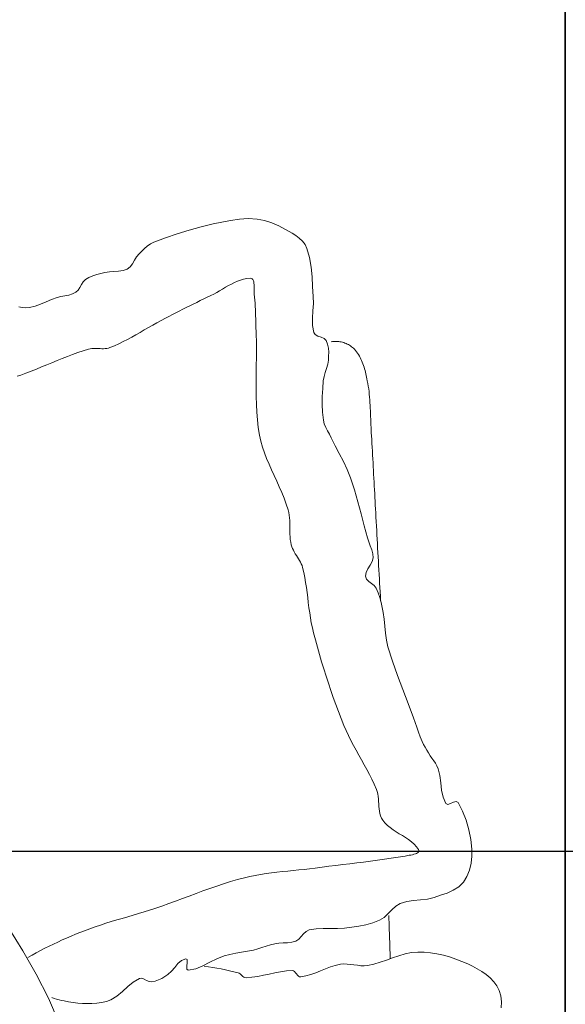
# Model space of a CAD drawing. Units: inches. Extents: x 1484 to 2008, y 1843 to 2590.
# Tile 8 of 21: x 1872 to 1891, y 2005 to 2040. Entities that reach past the tile are written whole.
import ezdxf

# ---------------------------------------------------------------- set-up
doc = ezdxf.new("R2010")
doc.units = ezdxf.units.IN
for name, color, linetype, lineweight in [('A-ANNO-DIMS', 2, 'Continuous', 18), ('A-FURN', 8, 'Continuous', 18), ('A-WALL', 7, 'Continuous', 35)]:
    doc.layers.add(name, color=color, linetype=linetype, lineweight=lineweight)
doc.styles.get("Standard").update_dxf_attribs({"font": 'arial.ttf'})
doc.dimstyles.new('ISO-25', dxfattribs={"dimtxt": 7, "dimasz": 2.5, "dimexe": 1.25, "dimexo": 0.625, "dimtad": 1, "dimdec": 0, "dimlunit": 3, "dimtxsty": 'Standard', "dimcen": 2.5, "dimadec": 0, "dimazin": 0, "dimtfac": 1, "dimtdec": 0, "dimtmove": 0, "dimatfit": 3, "dimfxl": 1, "dimarcsym": 0})

# ---------------------------------------------------------------- blocks, each defined once
blk = doc.blocks.new('BED-DOUBLE')
for p, q in [((28.429, 84.304), (28.269, 84.221)), ((28.626, 84.36), (28.429, 84.304)), ((28.83, 84.378), (28.626, 84.36)), ((29.039, 84.367), (28.83, 84.378)), ((27.993, 83.987), (27.874, 83.843)), ((28.125, 84.114), (27.993, 83.987)), ((28.269, 84.221), (28.125, 84.114)), ((27.767, 83.688), (27.669, 83.525)), ((27.874, 83.843), (27.767, 83.688)), ((22.439, 83.14), (22.774, 83.237)), ((22.774, 83.237), (23.115, 83.305)), ((23.115, 83.305), (23.459, 83.342)), ((23.459, 83.342), (23.703, 83.345)), ((23.703, 83.345), (23.949, 83.319)), ((23.949, 83.319), (24.19, 83.261)), ((24.19, 83.261), (24.417, 83.169)), ((27.581, 83.359), (27.5, 83.194)), ((27.669, 83.525), (27.581, 83.359)), ((21.807, 82.857), (22.115, 83.013)), ((22.115, 83.013), (22.439, 83.14)), ((24.417, 83.169), (24.62, 83.041)), ((24.62, 83.041), (24.781, 82.878)), ((27.408, 82.986), (27.325, 82.774)), ((27.5, 83.194), (27.408, 82.986)), ((21.775, 82.793), (21.807, 82.857)), ((21.804, 82.697), (21.775, 82.793)), ((21.852, 82.592), (21.804, 82.697)), ((21.881, 82.496), (21.852, 82.592)), ((24.781, 82.878), (24.905, 82.683)), ((24.905, 82.683), (25.002, 82.466)), ((27.253, 82.557), (27.191, 82.337)), ((27.325, 82.774), (27.253, 82.557)), ((20.621, 82.153), (20.867, 82.211)), ((20.867, 82.211), (21.122, 82.245)), ((21.122, 82.245), (21.376, 82.277)), ((21.376, 82.277), (21.622, 82.331)), ((21.622, 82.331), (21.85, 82.43)), ((21.85, 82.43), (21.881, 82.496)), ((25.002, 82.466), (25.082, 82.24)), ((25.082, 82.24), (25.156, 82.016)), ((27.191, 82.337), (27.142, 82.113)), ((20.067, 81.817), (20.166, 81.878)), ((20.166, 81.878), (20.256, 81.936)), ((20.256, 81.936), (20.344, 81.998)), ((20.344, 81.998), (20.432, 82.058)), ((20.432, 82.058), (20.524, 82.112)), ((20.524, 82.112), (20.621, 82.153)), ((25.156, 82.016), (25.212, 81.78)), ((27.107, 81.889), (27.086, 81.663)), ((27.142, 82.113), (27.107, 81.889)), ((19.333, 81.457), (19.499, 81.518)), ((19.499, 81.518), (19.662, 81.586)), ((19.662, 81.586), (19.767, 81.637)), ((19.767, 81.637), (19.868, 81.694)), ((19.868, 81.694), (19.968, 81.755)), ((19.968, 81.755), (20.067, 81.817)), ((25.212, 81.78), (25.241, 81.536)), ((25.241, 81.536), (25.262, 81.291)), ((27.086, 81.663), (27.081, 81.437)), ((18.331, 81.099), (18.829, 81.285)), ((18.829, 81.285), (18.997, 81.343)), ((18.997, 81.343), (19.165, 81.4)), ((19.165, 81.4), (19.333, 81.457)), ((23.12, 81.113), (23.197, 81.214)), ((23.197, 81.214), (23.28, 81.307)), ((23.28, 81.307), (23.371, 81.391)), ((23.371, 81.391), (23.472, 81.464)), ((23.472, 81.464), (23.504, 81.477)), ((23.504, 81.477), (23.533, 81.475)), ((23.533, 81.475), (23.559, 81.459)), ((23.559, 81.459), (23.582, 81.432)), ((23.582, 81.432), (23.603, 81.395)), ((23.603, 81.395), (23.621, 81.351)), ((23.621, 81.351), (23.637, 81.301)), ((23.637, 81.301), (23.65, 81.248)), ((23.65, 81.248), (23.662, 81.193)), ((23.662, 81.193), (23.673, 81.137)), ((25.262, 81.291), (25.297, 81.049)), ((27.081, 81.437), (27.1, 81.21)), ((27.1, 81.21), (27.146, 80.988)), ((17.338, 80.72), (17.835, 80.908)), ((17.835, 80.908), (18.331, 81.099)), ((22.912, 80.787), (22.98, 80.898)), ((22.98, 80.898), (23.048, 81.007)), ((23.048, 81.007), (23.12, 81.113)), ((23.673, 81.137), (23.682, 81.084)), ((23.682, 81.084), (23.69, 81.035)), ((23.69, 81.035), (23.698, 80.992)), ((23.698, 80.992), (23.739, 80.749)), ((25.297, 81.049), (25.366, 80.818)), ((25.366, 80.818), (25.462, 80.659)), ((27.146, 80.988), (27.21, 80.768)), ((16.33, 80.384), (16.837, 80.542)), ((16.837, 80.542), (17.338, 80.72)), ((22.618, 80.369), (22.698, 80.466)), ((22.698, 80.466), (22.773, 80.569)), ((22.773, 80.569), (22.844, 80.677)), ((22.844, 80.677), (22.912, 80.787)), ((23.739, 80.749), (23.778, 80.506)), ((23.778, 80.506), (23.814, 80.263)), ((25.462, 80.659), (25.591, 80.52)), ((25.591, 80.52), (25.731, 80.387)), ((26.936, 80.457), (27.013, 80.459)), ((27.013, 80.459), (27.09, 80.462)), ((27.09, 80.462), (27.166, 80.465)), ((27.166, 80.465), (27.243, 80.468)), ((27.21, 80.768), (27.285, 80.55)), ((27.243, 80.468), (27.319, 80.47)), ((27.285, 80.55), (27.365, 80.332)), ((14.241, 80.104), (14.395, 80.112)), ((14.395, 80.112), (14.55, 80.121)), ((14.55, 80.121), (14.705, 80.13)), ((14.594, 80.099), (14.766, 80.146)), ((14.766, 80.146), (14.94, 80.187)), ((14.94, 80.187), (15.115, 80.222)), ((15.115, 80.222), (15.357, 80.259)), ((15.357, 80.259), (15.602, 80.281)), ((15.602, 80.281), (15.848, 80.302)), ((15.848, 80.302), (16.091, 80.332)), ((16.091, 80.332), (16.33, 80.384)), ((22.204, 80.103), (22.283, 80.127)), ((22.283, 80.127), (22.36, 80.16)), ((22.36, 80.16), (22.432, 80.203)), ((22.432, 80.203), (22.529, 80.281)), ((22.529, 80.281), (22.618, 80.369)), ((23.814, 80.263), (23.848, 80.019)), ((25.731, 80.387), (25.862, 80.249)), ((25.788, 80.416), (25.865, 80.419)), ((25.862, 80.249), (25.961, 80.091)), ((25.865, 80.419), (25.941, 80.422)), ((25.941, 80.422), (26.018, 80.424)), ((26.018, 80.424), (26.094, 80.427)), ((26.094, 80.427), (26.171, 80.43)), ((26.171, 80.43), (26.247, 80.433)), ((26.247, 80.433), (26.324, 80.435)), ((26.324, 80.435), (26.401, 80.438)), ((26.401, 80.438), (26.477, 80.441)), ((26.477, 80.441), (26.554, 80.443)), ((26.554, 80.443), (26.63, 80.446)), ((26.63, 80.446), (26.707, 80.449)), ((26.707, 80.449), (26.783, 80.451)), ((26.783, 80.451), (26.86, 80.454)), ((26.86, 80.454), (26.936, 80.457)), ((27.365, 80.332), (27.441, 80.113)), ((27.441, 80.113), (27.506, 79.892)), ((7.824, 79.761), (7.921, 79.766)), ((7.921, 79.766), (8.019, 79.77)), ((8.019, 79.77), (8.116, 79.774)), ((8.116, 79.774), (8.214, 79.778)), ((8.214, 79.778), (8.311, 79.781)), ((8.311, 79.781), (8.409, 79.785)), ((8.409, 79.785), (8.506, 79.788)), ((8.506, 79.788), (8.604, 79.792)), ((8.604, 79.792), (8.701, 79.797)), ((8.701, 79.797), (8.798, 79.802)), ((8.798, 79.802), (8.896, 79.807)), ((8.896, 79.807), (9.031, 79.816)), ((9.031, 79.816), (9.167, 79.824)), ((9.167, 79.824), (9.303, 79.832)), ((9.303, 79.832), (9.439, 79.84)), ((9.439, 79.84), (9.574, 79.848)), ((9.574, 79.848), (9.71, 79.855)), ((9.71, 79.855), (9.846, 79.863)), ((9.846, 79.863), (9.982, 79.87)), ((9.982, 79.87), (10.117, 79.877)), ((10.117, 79.877), (10.253, 79.884)), ((10.253, 79.884), (10.389, 79.891)), ((10.389, 79.891), (10.525, 79.898)), ((10.525, 79.898), (10.661, 79.905)), ((10.661, 79.905), (10.796, 79.912)), ((10.796, 79.912), (10.932, 79.92)), ((10.932, 79.92), (11.068, 79.927)), ((11.068, 79.927), (11.204, 79.934)), ((11.204, 79.934), (11.339, 79.941)), ((11.339, 79.941), (11.475, 79.948)), ((11.475, 79.948), (11.611, 79.956)), ((11.611, 79.956), (11.766, 79.964)), ((11.766, 79.964), (11.92, 79.973)), ((11.92, 79.973), (12.075, 79.982)), ((12.075, 79.982), (12.23, 79.99)), ((12.23, 79.99), (12.385, 79.999)), ((12.385, 79.999), (12.539, 80.008)), ((12.539, 80.008), (12.694, 80.016)), ((12.631, 79.711), (12.771, 79.766)), ((12.694, 80.016), (12.849, 80.025)), ((12.771, 79.766), (12.91, 79.817)), ((12.849, 80.025), (13.003, 80.034)), ((12.91, 79.817), (13.051, 79.853)), ((13.003, 80.034), (13.158, 80.042)), ((13.051, 79.853), (13.195, 79.863)), ((13.158, 80.042), (13.313, 80.051)), ((13.195, 79.863), (13.33, 79.829)), ((13.313, 80.051), (13.467, 80.06)), ((13.33, 79.829), (13.458, 79.758)), ((13.467, 80.06), (13.622, 80.069)), ((13.622, 80.069), (13.777, 80.077)), ((13.777, 80.077), (13.931, 80.086)), ((13.931, 80.086), (14.086, 80.095)), ((14.024, 79.714), (14.097, 79.81)), ((14.086, 80.095), (14.241, 80.104)), ((14.097, 79.81), (14.174, 79.902)), ((14.174, 79.902), (14.264, 79.971)), ((14.264, 79.971), (14.426, 80.042)), ((14.426, 80.042), (14.594, 80.099)), ((20.823, 79.732), (20.996, 79.819)), ((20.996, 79.819), (21.172, 79.902)), ((21.172, 79.902), (21.349, 79.979)), ((21.349, 79.979), (21.43, 80.007)), ((21.43, 80.007), (21.513, 80.027)), ((21.513, 80.027), (21.598, 80.04)), ((21.598, 80.04), (21.685, 80.05)), ((21.685, 80.05), (21.773, 80.056)), ((21.773, 80.056), (21.861, 80.061)), ((21.861, 80.061), (21.949, 80.067)), ((21.949, 80.067), (22.036, 80.075)), ((22.036, 80.075), (22.121, 80.086)), ((22.121, 80.086), (22.204, 80.103)), ((23.848, 80.019), (23.88, 79.776)), ((23.88, 79.776), (23.911, 79.531)), ((25.961, 80.091), (26.05, 79.856)), ((26.05, 79.856), (26.116, 79.613)), ((27.506, 79.892), (27.553, 79.668)), ((6.14, 79.409), (6.194, 79.436)), ((6.194, 79.436), (6.25, 79.461)), ((6.25, 79.461), (6.306, 79.485)), ((6.306, 79.485), (6.363, 79.506)), ((6.363, 79.506), (6.421, 79.527)), ((6.421, 79.527), (6.479, 79.546)), ((6.479, 79.546), (6.538, 79.563)), ((6.538, 79.563), (6.598, 79.58)), ((6.598, 79.58), (6.657, 79.596)), ((6.657, 79.596), (6.717, 79.61)), ((6.717, 79.61), (6.777, 79.624)), ((6.777, 79.624), (6.836, 79.637)), ((6.836, 79.637), (6.896, 79.649)), ((6.896, 79.649), (6.955, 79.661)), ((6.955, 79.661), (7.05, 79.679)), ((7.05, 79.679), (7.146, 79.695)), ((7.146, 79.695), (7.242, 79.709)), ((7.242, 79.709), (7.339, 79.721)), ((7.339, 79.721), (7.436, 79.731)), ((7.436, 79.731), (7.532, 79.74)), ((7.532, 79.74), (7.629, 79.748)), ((7.629, 79.748), (7.726, 79.755)), ((7.726, 79.755), (7.824, 79.761)), ((11.218, 79.329), (11.642, 79.44)), ((11.642, 79.44), (12.068, 79.55)), ((12.068, 79.55), (12.492, 79.664)), ((12.492, 79.664), (12.631, 79.711)), ((13.458, 79.758), (13.583, 79.678)), ((13.583, 79.678), (13.71, 79.616)), ((13.71, 79.616), (13.844, 79.598)), ((13.844, 79.598), (13.943, 79.636)), ((13.943, 79.636), (14.024, 79.714)), ((20.143, 79.358), (20.312, 79.453)), ((20.312, 79.453), (20.482, 79.548)), ((20.482, 79.548), (20.652, 79.641)), ((20.652, 79.641), (20.823, 79.732)), ((23.911, 79.531), (23.941, 79.287)), ((26.116, 79.613), (26.165, 79.364)), ((27.56, 79.43), (27.547, 79.31)), ((27.553, 79.668), (27.563, 79.55)), ((27.563, 79.55), (27.56, 79.43)), ((5.708, 79.036), (5.732, 79.074)), ((5.732, 79.074), (5.758, 79.109)), ((5.758, 79.109), (5.786, 79.143)), ((5.786, 79.143), (5.815, 79.176)), ((5.815, 79.176), (5.845, 79.206)), ((5.845, 79.206), (5.89, 79.245)), ((5.89, 79.245), (5.937, 79.282)), ((5.937, 79.282), (5.986, 79.317)), ((5.986, 79.317), (6.036, 79.35)), ((6.036, 79.35), (6.087, 79.381)), ((6.087, 79.381), (6.14, 79.409)), ((10.38, 79.069), (10.796, 79.207)), ((10.796, 79.207), (11.218, 79.329)), ((19.457, 78.993), (19.631, 79.08)), ((19.631, 79.08), (19.802, 79.17)), ((19.802, 79.17), (19.973, 79.263)), ((19.973, 79.263), (20.143, 79.358)), ((23.941, 79.287), (23.97, 79.043)), ((26.165, 79.364), (26.203, 79.113)), ((26.203, 79.113), (26.238, 78.862)), ((27.53, 79.19), (27.513, 79.069)), ((27.547, 79.31), (27.53, 79.19)), ((5.583, 78.699), (5.591, 78.743)), ((5.591, 78.743), (5.602, 78.787)), ((5.602, 78.787), (5.615, 78.831)), ((5.615, 78.831), (5.63, 78.874)), ((5.63, 78.874), (5.647, 78.916)), ((5.647, 78.916), (5.665, 78.957)), ((5.665, 78.957), (5.686, 78.997)), ((5.686, 78.997), (5.708, 79.036)), ((9.525, 78.675), (9.805, 78.818)), ((9.805, 78.818), (10.089, 78.952)), ((10.089, 78.952), (10.38, 79.069)), ((18.61, 78.645), (18.857, 78.739)), ((18.857, 78.739), (19.103, 78.836)), ((19.103, 78.836), (19.282, 78.912)), ((19.282, 78.912), (19.457, 78.993)), ((23.97, 79.043), (23.999, 78.798)), ((23.999, 78.798), (24.028, 78.554)), ((26.238, 78.862), (26.256, 78.612)), ((27.501, 78.95), (27.499, 78.83)), ((27.499, 78.83), (27.51, 78.712)), ((27.513, 79.069), (27.501, 78.95)), ((5.57, 78.565), (5.572, 78.61)), ((5.57, 78.521), (5.57, 78.565)), ((5.573, 78.477), (5.57, 78.521)), ((5.572, 78.61), (5.576, 78.654)), ((5.578, 78.434), (5.573, 78.477)), ((5.576, 78.654), (5.583, 78.699)), ((5.585, 78.392), (5.578, 78.434)), ((8.842, 78.329), (8.963, 78.392)), ((8.963, 78.392), (9.245, 78.531)), ((9.245, 78.531), (9.525, 78.675)), ((17.611, 78.292), (17.862, 78.377)), ((17.862, 78.377), (18.112, 78.464)), ((18.112, 78.464), (18.362, 78.553)), ((18.362, 78.553), (18.61, 78.645)), ((24.028, 78.554), (24.058, 78.31)), ((26.256, 78.612), (26.254, 78.359)), ((27.51, 78.712), (27.551, 78.534)), ((27.551, 78.534), (27.606, 78.36)), ((5.383, 77.925), (5.421, 78.035)), ((5.421, 78.035), (5.467, 78.138)), ((5.467, 78.138), (5.54, 78.21)), ((5.54, 78.21), (5.668, 78.261)), ((5.668, 78.261), (5.805, 78.29)), ((5.805, 78.29), (5.946, 78.301)), ((5.946, 78.301), (6.089, 78.3)), ((6.089, 78.3), (6.23, 78.292)), ((6.23, 78.292), (6.378, 78.269)), ((6.378, 78.269), (6.523, 78.228)), ((6.523, 78.228), (6.667, 78.18)), ((6.667, 78.18), (6.812, 78.138)), ((6.812, 78.138), (6.959, 78.112)), ((6.959, 78.112), (7.236, 78.091)), ((7.236, 78.091), (7.514, 78.077)), ((7.514, 78.077), (7.791, 78.074)), ((7.791, 78.074), (8.068, 78.085)), ((8.068, 78.085), (8.344, 78.113)), ((8.344, 78.113), (8.475, 78.145)), ((8.475, 78.145), (8.6, 78.197)), ((8.6, 78.197), (8.721, 78.261)), ((8.721, 78.261), (8.842, 78.329)), ((16.599, 77.979), (16.853, 78.054)), ((16.853, 78.054), (17.107, 78.131)), ((17.107, 78.131), (17.359, 78.21)), ((17.359, 78.21), (17.611, 78.292)), ((24.058, 78.31), (24.089, 78.066)), ((24.089, 78.066), (24.121, 77.822)), ((26.254, 78.359), (26.249, 78.107)), ((26.249, 78.107), (26.259, 77.856)), ((27.606, 78.36), (27.671, 78.188)), ((27.671, 78.188), (27.74, 78.018)), ((2.959, 77.681), (3.3, 77.714)), ((3.3, 77.714), (3.644, 77.737)), ((3.644, 77.737), (3.985, 77.76)), ((3.985, 77.76), (4.24, 77.763)), ((4.24, 77.763), (4.497, 77.746)), ((4.497, 77.746), (4.753, 77.728)), ((4.753, 77.728), (5.007, 77.731)), ((5.007, 77.731), (5.254, 77.774)), ((5.254, 77.774), (5.333, 77.83)), ((5.333, 77.83), (5.383, 77.925)), ((15.308, 77.659), (15.484, 77.69)), ((15.484, 77.69), (15.659, 77.726)), ((15.659, 77.726), (15.833, 77.768)), ((15.833, 77.768), (16.089, 77.836)), ((16.089, 77.836), (16.344, 77.906)), ((16.344, 77.906), (16.599, 77.979)), ((24.121, 77.822), (24.145, 77.631)), ((26.259, 77.856), (26.301, 77.611)), ((27.74, 78.018), (27.809, 77.847)), ((27.809, 77.847), (27.871, 77.675)), ((1.936, 77.268), (2.041, 77.381)), ((2.041, 77.381), (2.16, 77.473)), ((2.16, 77.473), (2.294, 77.537)), ((2.294, 77.537), (2.622, 77.626)), ((2.622, 77.626), (2.959, 77.681)), ((13.345, 77.308), (13.407, 77.338)), ((13.407, 77.338), (13.47, 77.363)), ((13.47, 77.363), (13.536, 77.383)), ((13.536, 77.383), (13.71, 77.423)), ((13.71, 77.423), (13.886, 77.458)), ((13.886, 77.458), (14.062, 77.489)), ((14.062, 77.489), (14.24, 77.515)), ((14.24, 77.515), (14.418, 77.54)), ((14.418, 77.54), (14.596, 77.562)), ((14.596, 77.562), (14.774, 77.584)), ((14.774, 77.584), (14.953, 77.607)), ((14.953, 77.607), (15.13, 77.632)), ((15.13, 77.632), (15.308, 77.659)), ((24.145, 77.631), (24.167, 77.439)), ((24.167, 77.439), (24.188, 77.247)), ((26.301, 77.611), (26.354, 77.505)), ((26.354, 77.505), (26.439, 77.416)), ((26.439, 77.416), (26.536, 77.332)), ((27.871, 77.675), (27.922, 77.5)), ((27.922, 77.5), (27.956, 77.322)), ((1.63, 76.781), (1.762, 77.014)), ((1.762, 77.014), (1.843, 77.143)), ((1.843, 77.143), (1.936, 77.268)), ((12.738, 76.984), (12.803, 77.004)), ((12.803, 77.004), (12.867, 77.029)), ((12.867, 77.029), (12.929, 77.059)), ((12.929, 77.059), (12.989, 77.092)), ((12.989, 77.092), (13.049, 77.127)), ((13.049, 77.127), (13.108, 77.164)), ((13.108, 77.164), (13.166, 77.202)), ((13.166, 77.202), (13.225, 77.239)), ((13.225, 77.239), (13.285, 77.275)), ((13.285, 77.275), (13.345, 77.308)), ((24.188, 77.247), (24.207, 77.055)), ((24.207, 77.055), (24.226, 76.863)), ((26.536, 77.332), (26.627, 77.245)), ((26.627, 77.245), (26.692, 77.143)), ((26.692, 77.143), (26.733, 77.001)), ((26.733, 77.001), (26.753, 76.853)), ((27.743, 77.064), (27.733, 77.02)), ((27.733, 77.02), (27.745, 76.815)), ((27.769, 77.102), (27.743, 77.064)), ((27.807, 77.138), (27.769, 77.102)), ((27.85, 77.171), (27.807, 77.138)), ((27.892, 77.205), (27.85, 77.171)), ((27.928, 77.24), (27.892, 77.205)), ((27.951, 77.278), (27.928, 77.24)), ((27.956, 77.322), (27.951, 77.278)), ((1.506, 76.542), (1.63, 76.781)), ((10.694, 76.563), (10.894, 76.65)), ((10.894, 76.65), (11.095, 76.732)), ((11.095, 76.732), (11.299, 76.806)), ((11.299, 76.806), (11.505, 76.872)), ((11.505, 76.872), (11.597, 76.894)), ((11.597, 76.894), (11.69, 76.911)), ((11.69, 76.911), (11.785, 76.922)), ((11.785, 76.922), (11.88, 76.928)), ((11.88, 76.928), (11.976, 76.931)), ((11.976, 76.931), (12.072, 76.933)), ((12.072, 76.933), (12.168, 76.933)), ((12.168, 76.933), (12.265, 76.934)), ((12.265, 76.934), (12.361, 76.937)), ((12.361, 76.937), (12.456, 76.942)), ((12.456, 76.942), (12.551, 76.951)), ((12.551, 76.951), (12.645, 76.964)), ((12.645, 76.964), (12.738, 76.984)), ((24.226, 76.863), (24.246, 76.671)), ((24.246, 76.671), (24.267, 76.479)), ((26.753, 76.853), (26.761, 76.702)), ((26.761, 76.702), (26.771, 76.552)), ((27.745, 76.815), (27.773, 76.611)), ((1.315, 76.042), (1.398, 76.295)), ((1.398, 76.295), (1.506, 76.542)), ((10.1, 76.29), (10.298, 76.381)), ((10.298, 76.381), (10.496, 76.473)), ((10.496, 76.473), (10.694, 76.563)), ((24.267, 76.479), (24.29, 76.288)), ((26.771, 76.552), (26.792, 76.404)), ((26.792, 76.404), (26.83, 76.252)), ((27.773, 76.611), (27.811, 76.409)), ((27.811, 76.409), (27.854, 76.207)), ((1.265, 75.782), (1.315, 76.042)), ((9.087, 75.914), (9.295, 75.972)), ((9.295, 75.972), (9.499, 76.041)), ((9.499, 76.041), (9.701, 76.118)), ((9.701, 76.118), (9.901, 76.202)), ((9.901, 76.202), (10.1, 76.29)), ((24.29, 76.288), (24.316, 76.097)), ((24.316, 76.097), (24.346, 75.907)), ((26.83, 76.252), (26.874, 76.101)), ((26.874, 76.101), (26.922, 75.952)), ((26.922, 75.952), (26.968, 75.802)), ((27.854, 76.207), (27.899, 76.005)), ((27.899, 76.005), (27.939, 75.803)), ((1.249, 75.472), (1.265, 75.782)), ((3.352, 75.576), (3.369, 75.608)), ((3.369, 75.608), (3.397, 75.632)), ((3.397, 75.632), (3.433, 75.65)), ((3.433, 75.65), (3.476, 75.662)), ((3.476, 75.662), (3.525, 75.67)), ((3.525, 75.67), (3.579, 75.675)), ((3.579, 75.675), (3.635, 75.677)), ((3.635, 75.677), (3.693, 75.677)), ((3.693, 75.677), (3.75, 75.677)), ((3.75, 75.677), (3.805, 75.677)), ((3.805, 75.677), (3.857, 75.678)), ((3.857, 75.678), (3.904, 75.682)), ((3.904, 75.682), (4.013, 75.692)), ((4.013, 75.692), (4.121, 75.701)), ((4.121, 75.701), (4.23, 75.709)), ((4.23, 75.709), (4.339, 75.716)), ((4.339, 75.716), (4.448, 75.721)), ((4.448, 75.721), (4.557, 75.726)), ((4.557, 75.726), (4.666, 75.729)), ((4.666, 75.729), (4.775, 75.733)), ((4.775, 75.733), (4.884, 75.736)), ((4.884, 75.736), (4.993, 75.739)), ((4.993, 75.739), (5.102, 75.742)), ((5.102, 75.742), (5.211, 75.745)), ((5.211, 75.745), (5.32, 75.749)), ((5.32, 75.749), (5.594, 75.756)), ((5.594, 75.756), (5.868, 75.759)), ((5.868, 75.759), (6.143, 75.757)), ((6.143, 75.757), (6.418, 75.754)), ((6.418, 75.754), (6.693, 75.75)), ((6.693, 75.75), (6.967, 75.747)), ((6.967, 75.747), (7.242, 75.746)), ((7.242, 75.746), (7.516, 75.749)), ((7.516, 75.749), (7.79, 75.757)), ((7.79, 75.757), (8.063, 75.771)), ((8.063, 75.771), (8.335, 75.794)), ((8.335, 75.794), (8.606, 75.825)), ((8.606, 75.825), (8.876, 75.868)), ((8.876, 75.868), (9.087, 75.914)), ((24.346, 75.907), (24.379, 75.717)), ((24.379, 75.717), (24.417, 75.529)), ((26.968, 75.802), (27.008, 75.651)), ((27.008, 75.651), (27.051, 75.444)), ((27.939, 75.803), (27.97, 75.599)), ((1.266, 75.162), (1.249, 75.472)), ((3.347, 75.536), (3.352, 75.576)), ((3.358, 75.421), (3.347, 75.536)), ((3.379, 75.308), (3.358, 75.421)), ((3.411, 75.198), (3.379, 75.308)), ((24.417, 75.529), (24.461, 75.342)), ((24.461, 75.342), (24.527, 75.094)), ((27.051, 75.444), (27.086, 75.236)), ((27.941, 75.284), (27.912, 75.251)), ((27.966, 75.318), (27.941, 75.284)), ((27.982, 75.355), (27.966, 75.318)), ((27.97, 75.599), (27.987, 75.395)), ((27.987, 75.395), (27.982, 75.355)), ((1.309, 74.851), (1.266, 75.162)), ((3.451, 75.09), (3.411, 75.198)), ((3.498, 74.983), (3.451, 75.09)), ((3.551, 74.878), (3.498, 74.983)), ((24.527, 75.094), (24.599, 74.848)), ((27.086, 75.236), (27.12, 75.028)), ((27.12, 75.028), (27.161, 74.821)), ((27.773, 74.963), (27.737, 74.816)), ((27.812, 75.11), (27.773, 74.963)), ((27.829, 75.149), (27.812, 75.11)), ((27.853, 75.184), (27.829, 75.149)), ((27.882, 75.218), (27.853, 75.184)), ((27.912, 75.251), (27.882, 75.218)), ((1.368, 74.543), (1.309, 74.851)), ((3.607, 74.773), (3.551, 74.878)), ((3.667, 74.669), (3.607, 74.773)), ((3.728, 74.566), (3.667, 74.669)), ((3.789, 74.463), (3.728, 74.566)), ((24.599, 74.848), (24.676, 74.603)), ((24.676, 74.603), (24.757, 74.36)), ((27.161, 74.821), (27.215, 74.618)), ((27.215, 74.618), (27.316, 74.365)), ((27.703, 74.667), (27.672, 74.518)), ((27.737, 74.816), (27.703, 74.667)), ((1.435, 74.237), (1.368, 74.543)), ((1.537, 73.811), (1.435, 74.237)), ((3.849, 74.359), (3.789, 74.463)), ((3.906, 74.255), (3.849, 74.359)), ((3.958, 74.15), (3.906, 74.255)), ((24.757, 74.36), (24.842, 74.118)), ((27.316, 74.365), (27.442, 74.119)), ((27.619, 74.219), (27.597, 74.069)), ((27.644, 74.369), (27.619, 74.219)), ((27.672, 74.518), (27.644, 74.369)), ((4.017, 74.026), (3.958, 74.15)), ((4.076, 73.903), (4.017, 74.026)), ((4.136, 73.779), (4.076, 73.903)), ((24.842, 74.118), (24.929, 73.877)), ((24.929, 73.877), (25.018, 73.636)), ((27.442, 74.119), (27.569, 73.874)), ((27.569, 73.874), (27.67, 73.623)), ((27.597, 74.069), (27.578, 73.918)), ((1.652, 73.387), (1.537, 73.811)), ((4.196, 73.656), (4.136, 73.779)), ((4.257, 73.533), (4.196, 73.656)), ((4.319, 73.41), (4.257, 73.533)), ((25.018, 73.636), (25.108, 73.395)), ((27.67, 73.623), (27.723, 73.361)), ((1.78, 72.968), (1.652, 73.387)), ((4.38, 73.288), (4.319, 73.41)), ((4.442, 73.165), (4.38, 73.288)), ((25.108, 73.395), (25.198, 73.155)), ((27.346, 73.318), (27.313, 73.269)), ((27.313, 73.269), (27.378, 73.12)), ((27.448, 73.32), (27.346, 73.318)), ((27.575, 73.308), (27.448, 73.32)), ((27.682, 73.311), (27.575, 73.308)), ((27.723, 73.361), (27.682, 73.311)), ((1.922, 72.553), (1.78, 72.968)), ((4.504, 73.043), (4.442, 73.165)), ((4.567, 72.921), (4.504, 73.043)), ((4.629, 72.799), (4.567, 72.921)), ((25.198, 73.155), (25.288, 72.914)), ((25.288, 72.914), (25.375, 72.673)), ((27.378, 73.12), (27.489, 72.995)), ((27.489, 72.995), (27.624, 72.882)), ((27.624, 72.882), (27.759, 72.768)), ((2.079, 72.144), (1.922, 72.553)), ((4.692, 72.677), (4.629, 72.799)), ((4.755, 72.555), (4.692, 72.677)), ((4.834, 72.404), (4.755, 72.555)), ((25.375, 72.673), (25.461, 72.431)), ((27.759, 72.768), (27.872, 72.64)), ((27.872, 72.64), (27.942, 72.534)), ((27.942, 72.534), (28.007, 72.424)), ((2.138, 72.026), (2.079, 72.144)), ((4.916, 72.255), (4.834, 72.404)), ((5, 72.107), (4.916, 72.255)), ((25.461, 72.431), (25.543, 72.188)), ((25.543, 72.188), (25.605, 71.997)), ((28.007, 72.424), (28.063, 72.31)), ((28.063, 72.31), (28.107, 72.192)), ((28.107, 72.192), (28.134, 72.069)), ((2.213, 71.918), (2.138, 72.026)), ((2.299, 71.816), (2.213, 71.918)), ((2.392, 71.72), (2.299, 71.816)), ((5.084, 71.959), (5, 72.107)), ((5.17, 71.811), (5.084, 71.959)), ((5.255, 71.664), (5.17, 71.811)), ((25.605, 71.997), (25.665, 71.805)), ((25.665, 71.805), (25.723, 71.613)), ((28.035, 71.806), (28.004, 71.721)), ((28.082, 71.893), (28.035, 71.806)), ((28.123, 71.981), (28.082, 71.893)), ((28.134, 72.069), (28.123, 71.981)), ((2.487, 71.626), (2.392, 71.72)), ((2.594, 71.541), (2.487, 71.626)), ((2.715, 71.469), (2.594, 71.541)), ((2.835, 71.397), (2.715, 71.469)), ((5.339, 71.515), (5.255, 71.664)), ((5.422, 71.367), (5.339, 71.515)), ((25.723, 71.613), (25.78, 71.421)), ((28.004, 71.721), (28.012, 71.638)), ((28.012, 71.638), (28.137, 71.423)), ((2.942, 71.315), (2.835, 71.397)), ((3.024, 71.211), (2.942, 71.315)), ((3.079, 71.064), (3.024, 71.211)), ((5.502, 71.217), (5.422, 71.367)), ((5.58, 71.066), (5.502, 71.217)), ((25.78, 71.421), (25.837, 71.228)), ((25.837, 71.228), (25.893, 71.036)), ((28.137, 71.423), (28.296, 71.228)), ((28.296, 71.228), (28.468, 71.04)), ((3.102, 70.907), (3.079, 71.064)), ((3.11, 70.744), (3.102, 70.907)), ((5.655, 70.914), (5.58, 71.066)), ((5.725, 70.759), (5.655, 70.914)), ((5.791, 70.603), (5.725, 70.759)), ((25.893, 71.036), (25.95, 70.843)), ((25.95, 70.843), (26.008, 70.651)), ((28.468, 71.04), (28.63, 70.847)), ((28.63, 70.847), (28.762, 70.635)), ((3.118, 70.581), (3.11, 70.744)), ((3.142, 70.423), (3.118, 70.581)), ((3.177, 70.28), (3.142, 70.423)), ((5.809, 70.548), (5.791, 70.603)), ((5.821, 70.491), (5.809, 70.548)), ((5.827, 70.434), (5.821, 70.491)), ((5.83, 70.375), (5.827, 70.434)), ((26.008, 70.651), (26.067, 70.46)), ((26.067, 70.46), (26.128, 70.269)), ((28.762, 70.635), (28.822, 70.477)), ((28.822, 70.477), (28.86, 70.311)), ((3.215, 70.137), (3.177, 70.28)), ((3.26, 69.997), (3.215, 70.137)), ((5.817, 70.077), (5.819, 70.137)), ((5.817, 70.018), (5.817, 70.077)), ((5.819, 70.137), (5.822, 70.197)), ((5.822, 70.197), (5.826, 70.257)), ((5.826, 70.257), (5.829, 70.316)), ((5.829, 70.316), (5.83, 70.375)), ((26.128, 70.269), (26.192, 70.079)), ((26.192, 70.079), (26.259, 69.89)), ((28.86, 70.311), (28.882, 70.141)), ((28.882, 70.141), (28.892, 69.969)), ((3.317, 69.862), (3.26, 69.997)), ((3.39, 69.737), (3.317, 69.862)), ((3.468, 69.657), (3.39, 69.737)), ((5.82, 69.96), (5.817, 70.018)), ((5.829, 69.902), (5.82, 69.96)), ((5.842, 69.846), (5.829, 69.902)), ((5.902, 69.659), (5.842, 69.846)), ((26.259, 69.89), (26.329, 69.702)), ((28.892, 69.969), (28.897, 69.797)), ((28.897, 69.797), (28.894, 69.635)), ((3.566, 69.597), (3.468, 69.657)), ((3.67, 69.543), (3.566, 69.597)), ((3.767, 69.482), (3.67, 69.543)), ((3.843, 69.402), (3.767, 69.482)), ((3.902, 69.281), (3.843, 69.402)), ((5.966, 69.473), (5.902, 69.659)), ((6.033, 69.289), (5.966, 69.473)), ((26.329, 69.702), (26.391, 69.545)), ((26.391, 69.545), (26.454, 69.388)), ((26.454, 69.388), (26.52, 69.232)), ((28.88, 69.472), (28.858, 69.31)), ((28.894, 69.635), (28.88, 69.472)), ((3.939, 69.151), (3.902, 69.281)), ((3.965, 69.015), (3.939, 69.151)), ((3.99, 68.879), (3.965, 69.015)), ((6.103, 69.105), (6.033, 69.289)), ((6.175, 68.922), (6.103, 69.105)), ((26.52, 69.232), (26.587, 69.076)), ((26.587, 69.076), (26.655, 68.922)), ((28.83, 69.149), (28.802, 68.988)), ((28.858, 69.31), (28.83, 69.149)), ((4.024, 68.747), (3.99, 68.879)), ((4.096, 68.551), (4.024, 68.747)), ((6.248, 68.74), (6.175, 68.922)), ((6.323, 68.558), (6.248, 68.74)), ((26.655, 68.922), (26.726, 68.768)), ((26.726, 68.768), (26.798, 68.615)), ((29.579, 68.813), (28.71, 68.44)), ((28.739, 68.726), (28.712, 68.64)), ((28.764, 68.812), (28.739, 68.726)), ((28.785, 68.9), (28.764, 68.812)), ((28.802, 68.988), (28.785, 68.9)), ((4.176, 68.358), (4.096, 68.551)), ((4.256, 68.164), (4.176, 68.358)), ((6.398, 68.376), (6.323, 68.558)), ((6.472, 68.195), (6.398, 68.376)), ((26.798, 68.615), (26.872, 68.462)), ((26.872, 68.462), (26.948, 68.311)), ((28.71, 68.44), (27.864, 68.011)), ((28.712, 68.64), (28.68, 68.556)), ((4.326, 67.968), (4.256, 68.164)), ((6.546, 68.012), (6.472, 68.195)), ((6.619, 67.83), (6.546, 68.012)), ((26.948, 68.311), (27.025, 68.16)), ((27.025, 68.16), (27.104, 68.011)), ((27.864, 68.011), (27.04, 67.54)), ((27.104, 68.011), (27.185, 67.862)), ((4.377, 67.767), (4.326, 67.968)), ((4.375, 67.517), (4.386, 67.642)), ((4.386, 67.642), (4.377, 67.767)), ((6.689, 67.646), (6.619, 67.83)), ((6.757, 67.462), (6.689, 67.646)), ((27.185, 67.862), (27.267, 67.714)), ((4.353, 67.391), (4.375, 67.517)), ((6.802, 67.342), (6.757, 67.462)), ((27.04, 67.54), (26.237, 67.038))]:
    blk.add_line(p, q)
blk = doc.blocks.new('*D32')
at = {"layer": 'A-ANNO-DIMS', "color": 0, "lineweight": -2, "transparency": 16777216}
for p, q in [((1961.855, 2010.803), (1961.855, 2038.599)), ((1648.545, 2010.803), (1963.105, 2010.803)), ((1961.855, 2003.303), (1961.855, 2008.303)), ((1648.545, 2000.803), (1963.105, 2000.803))]:
    blk.add_line(p, q, dxfattribs=at)
at = {"layer": 'A-ANNO-DIMS', "color": 0, "transparency": 16777216}
for points in [[(1961.438, 2008.303), (1962.271, 2008.303), (1961.855, 2010.803)], [(1961.438, 2003.303), (1962.271, 2003.303), (1961.855, 2000.803)]]:
    blk.add_solid(points, dxfattribs=at)
at = {"layer": 'Defpoints', "color": 0, "transparency": 16777216}
for p in [(1647.92, 2010.803), (1961.855, 2010.803), (1647.92, 2000.803)]:
    blk.add_point(p, dxfattribs=at)
at = {"layer": 'A-ANNO-DIMS', "color": 0, "transparency": 16777216, "insert": (1957.656, 2025.951), "char_height": 7, "attachment_point": 5, "rotation": 90}
blk.add_mtext('0\'-10"', dxfattribs=at)

msp = doc.modelspace()

# ---------------------------------------------------------------- linework, layer by layer
at = {"layer": 'A-WALL'}
msp.add_line((1890.92, 2072.803), (1890.92, 1928.803), dxfattribs=at)

# ---------------------------------------------------------------- block references
at = {"layer": 'A-FURN', "rotation": 269.9999999999906}
msp.add_blockref('BED-DOUBLE', (1804.291, 2034.333), dxfattribs=at)

# ---------------------------------------------------------------- dimensions: what is measured, and where the dimension line sits
at = {"layer": 'A-ANNO-DIMS'}
dim = msp.add_linear_dim(base=(1961.855, 2010.803), p1=(1647.92, 2000.803), p2=(1647.92, 2010.803), angle=90, dimstyle='ISO-25', override={"dimdec": 1, "dimlfac": 1, "dimrnd": 0, "dimzin": 1, "dimdsep": 46, "dimlunit": 4, "dimfrac": 2}, dxfattribs=at)
dim.commit()
dim.dimension.update_dxf_attribs({"geometry": '*D32', "text_midpoint": (1957.656, 2025.951)})

doc.saveas('drawing.dxf')
